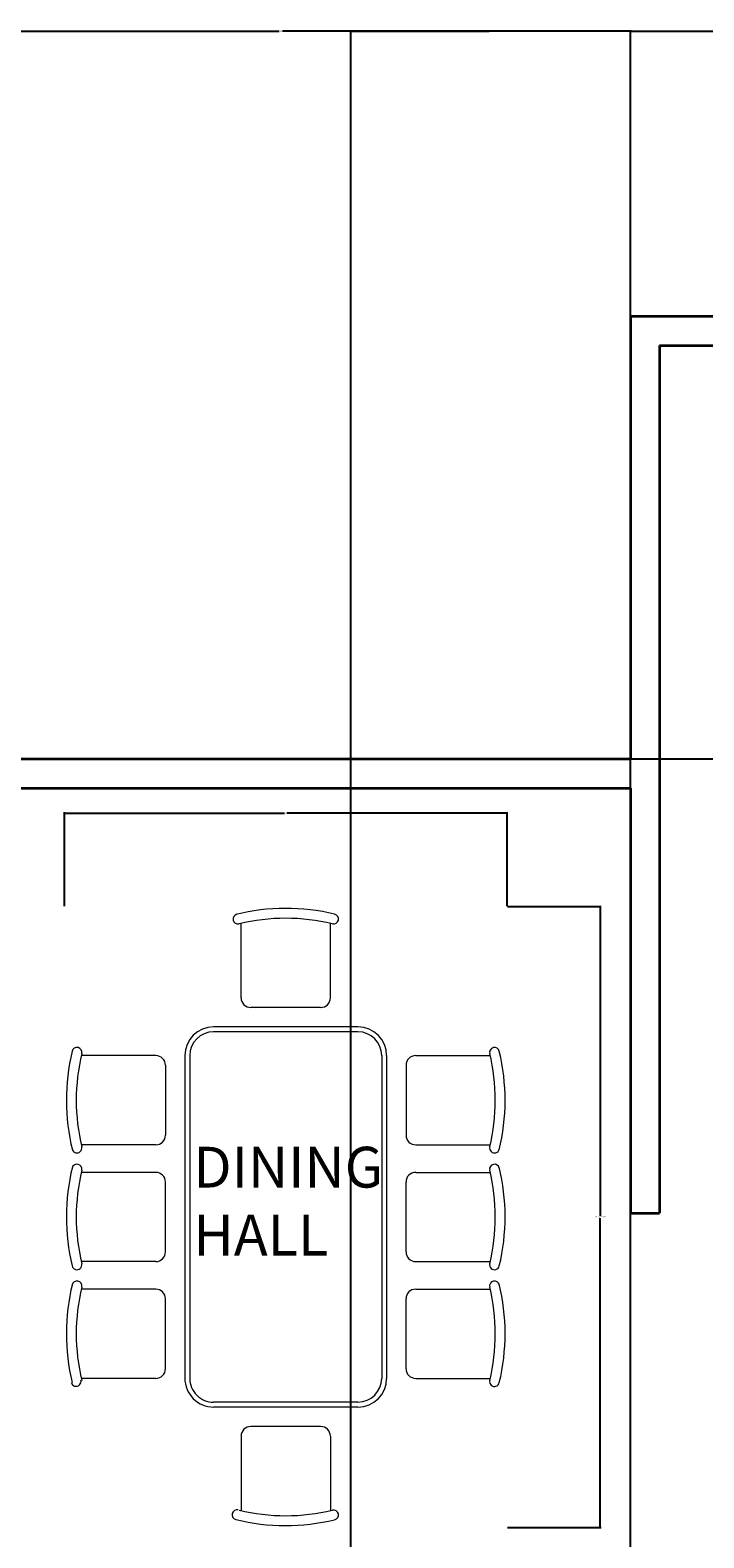
# Model space of a CAD drawing. Units: inches. Extents: x 3731 to 4318, y 1310 to 2388.
# Tile 49 of 57: x 4000 to 4116, y 2129 to 2388. Entities that reach past the tile are written whole.
import ezdxf

# ---------------------------------------------------------------- set-up
doc = ezdxf.new("R2010")
doc.units = ezdxf.units.IN
for name, color, linetype, lineweight in [('A-ANNO-DIMS', 2, 'Continuous', 18), ('A-AREA-IDEN', 7, 'Continuous', 18), ('A-FURN', 8, 'Continuous', 13), ('A-WALL', 7, 'Continuous', 35)]:
    doc.layers.add(name, color=color, linetype=linetype, lineweight=lineweight)
doc.styles.get("Standard").update_dxf_attribs({"font": 'arial.ttf'})
doc.dimstyles.get("Standard").update_dxf_attribs({"dimtxt": 0.18, "dimasz": 0.18, "dimexe": 0.18, "dimexo": 0.0625, "dimgap": 0.09, "dimtad": 0, "dimtih": 1, "dimtoh": 1, "dimdec": 4, "dimzin": 0, "dimdsep": 46, "dimtxsty": 'Standard', "dimcen": 0.09, "dimadec": 0, "dimazin": 0, "dimtfac": 1, "dimtdec": 4, "dimtofl": 0, "dimtmove": 0, "dimatfit": 3, "dimfxl": 1, "dimtolj": 1, "dimtzin": 0, "dimarcsym": 0})

# ---------------------------------------------------------------- blocks, each defined once
blk = doc.blocks.new('A$C593F2FDE')
for p, q in [((0.8501, 2.0223), (0.8501, 2.4542)), ((1.3676, 2.0223), (1.3676, 2.4542)), ((1.5273, 2.0223), (1.5273, 2.4542)), ((2.0448, 2.0223), (2.0448, 2.4542)), ((2.2045, 2.0223), (2.2045, 2.4542)), ((2.722, 2.0223), (2.722, 2.4542)), ((0.9063, 1.966), (1.3113, 1.966)), ((1.9885, 1.966), (1.5835, 1.966)), ((2.6658, 1.966), (2.2608, 1.966)), ((0.85, 1.8535), (2.722, 1.8535)), ((0.85, 1.825), (2.722, 1.825)), ((0.6835, 1.687), (0.6835, 0.85)), ((0.7121, 1.687), (0.7121, 0.85)), ((2.86, 1.687), (2.86, 0.85)), ((2.8885, 1.687), (2.8885, 0.85)), ((0.5148, 1.5273), (0.0828, 1.5273)), ((3.0573, 1.5273), (3.4892, 1.5273)), ((0.571, 1.471), (0.571, 1.066)), ((3.001, 1.471), (3.001, 1.066)), ((0.5148, 1.0098), (0.0828, 1.0098)), ((3.0573, 1.0098), (3.4892, 1.0098)), ((0.85, 0.7121), (2.722, 0.7121)), ((0.85, 0.6835), (2.722, 0.6835)), ((0.9063, 0.571), (1.3113, 0.571)), ((1.9885, 0.571), (1.5835, 0.571)), ((2.6658, 0.571), (2.2608, 0.571)), ((0.8501, 0.5148), (0.8501, 0.0828)), ((1.3676, 0.5148), (1.3676, 0.0828)), ((1.5273, 0.5148), (1.5273, 0.0828)), ((2.0448, 0.5148), (2.0448, 0.0828)), ((2.2045, 0.5148), (2.2045, 0.0828)), ((2.722, 0.5148), (2.722, 0.0828))]:
    blk.add_line(p, q)
for centre, radius, start, end in [((1.1088, 1.3263), 1.2144, 76.2483, 103.50545), ((1.786, 1.3263), 1.2144, 76.49455, 103.7517), ((2.4633, 1.3263), 1.2144, 76.49455, 103.7517), ((0.8316, 2.4793), 0.0286, 102.88207, 282.88207), ((1.1088, 1.3263), 1.1572, 76.46376, 103.53624), ((1.386, 2.4793), 0.0286, 257.11793, 77.11793), ((1.5088, 2.4793), 0.0286, 102.88207, 282.88207), ((1.786, 1.3263), 1.1572, 76.46376, 103.53624), ((2.0633, 2.4793), 0.0286, 257.11793, 77.11793), ((2.186, 2.4793), 0.0286, 102.88207, 282.88207), ((2.4633, 1.3263), 1.1572, 76.46376, 103.53624), ((2.7405, 2.4793), 0.0286, 257.11793, 77.11793), ((0.9063, 2.0223), 0.0563, 180, 270), ((1.3113, 2.0223), 0.0563, 270, 0), ((1.5835, 2.0223), 0.0563, 180, 270), ((1.9885, 2.0223), 0.0563, 270, 0), ((2.2608, 2.0223), 0.0563, 180, 270), ((2.6658, 2.0223), 0.0563, 270, 0), ((0.85, 1.687), 0.1665, 90, 180), ((2.722, 1.687), 0.1665, 0, 90), ((0.85, 1.687), 0.1379, 90, 180), ((2.722, 1.687), 0.1379, 0, 90), ((0.0578, 1.5458), 0.0286, 347.11793, 167.11793), ((3.5143, 1.5458), 0.0286, 12.88207, 192.88207), ((1.2108, 1.2685), 1.2144, 166.49455, 193.7517), ((1.2108, 1.2685), 1.1572, 166.46376, 193.53624), ((0.5148, 1.471), 0.0563, 0, 90), ((3.0573, 1.471), 0.0563, 90, 180), ((2.3613, 1.2685), 1.1572, 346.46376, 13.53624), ((2.3613, 1.2685), 1.2144, 346.2483, 13.50545), ((0.5148, 1.066), 0.0563, 270, 0), ((3.0573, 1.066), 0.0563, 180, 270), ((0.0578, 0.9913), 0.0286, 192.88207, 12.88207), ((3.513, 0.9862), 0.0286, 167.11793, 347.11793), ((0.85, 0.85), 0.1665, 180, 270), ((0.85, 0.85), 0.1379, 180, 270), ((2.722, 0.85), 0.1665, 270, 0), ((2.722, 0.85), 0.1379, 270, 0), ((0.9063, 0.5148), 0.0563, 90, 180), ((1.3113, 0.5148), 0.0563, 0, 90), ((1.5835, 0.5148), 0.0563, 90, 180), ((1.9885, 0.5148), 0.0563, 0, 90), ((2.2608, 0.5148), 0.0563, 90, 180), ((2.6658, 0.5148), 0.0563, 0, 90), ((0.8316, 0.0578), 0.0286, 77.11793, 257.11793), ((1.1088, 1.2108), 1.2144, 256.49455, 283.7517), ((1.1088, 1.2108), 1.1572, 256.46376, 283.53624), ((1.386, 0.0578), 0.0286, 282.88207, 102.88207), ((1.5088, 0.0578), 0.0286, 77.11793, 257.11793), ((1.786, 1.2108), 1.2144, 256.2483, 283.50545), ((1.786, 1.2108), 1.1572, 256.46376, 283.53624), ((2.0633, 0.0578), 0.0286, 282.88207, 102.88207), ((2.186, 0.0578), 0.0286, 77.11793, 257.11793), ((2.4633, 1.2108), 1.2144, 256.2483, 283.50545), ((2.4633, 1.2108), 1.1572, 256.46376, 283.53624), ((2.7393, 0.0528), 0.0286, 282.88207, 102.88207)]:
    blk.add_arc(centre, radius, start, end)
blk = doc.blocks.new('*D30')
at = {"layer": 'A-ANNO-DIMS', "color": 0, "lineweight": -2, "transparency": 16777216}
for p, q in [((4082.11, 2237.06), (4098.22, 2237.06)), ((4098.04, 2236.88), (4098.04, 2183.92)), ((4098.04, 2130.59), (4098.04, 2183.55)), ((4082.11, 2130.41), (4098.22, 2130.41))]:
    blk.add_line(p, q, dxfattribs=at)
at = {"layer": 'A-ANNO-DIMS', "color": 0, "transparency": 16777216}
for points in [[(4098.01, 2236.88), (4098.07, 2236.88), (4098.04, 2237.06)], [(4098.01, 2130.59), (4098.07, 2130.59), (4098.04, 2130.41)]]:
    blk.add_solid(points, dxfattribs=at)
at = {"layer": 'Defpoints', "color": 0, "transparency": 16777216}
for p in [(4082.05, 2237.06), (4082.05, 2130.41), (4098.04, 2130.41)]:
    blk.add_point(p, dxfattribs=at)
at = {"layer": 'A-ANNO-DIMS', "color": 0, "transparency": 16777216, "insert": (4098.04, 2183.74), "char_height": 0.18, "attachment_point": 5}
blk.add_mtext('\\A1;DINING SET 107', dxfattribs=at)
blk = doc.blocks.new('*D31')
at = {"layer": 'A-ANNO-DIMS', "color": 0, "lineweight": -2, "transparency": 16777216}
for p, q in [((4006.04, 2237.12), (4006.04, 2253.24)), ((4006.22, 2253.06), (4043.82, 2253.06)), ((4081.87, 2253.06), (4044.26, 2253.06)), ((4082.05, 2237.12), (4082.05, 2253.24))]:
    blk.add_line(p, q, dxfattribs=at)
at = {"layer": 'A-ANNO-DIMS', "color": 0, "transparency": 16777216}
for points in [[(4006.22, 2253.09), (4006.22, 2253.03), (4006.04, 2253.06)], [(4081.87, 2253.09), (4081.87, 2253.03), (4082.05, 2253.06)]]:
    blk.add_solid(points, dxfattribs=at)
at = {"layer": 'Defpoints', "color": 0, "transparency": 16777216}
for p in [(4082.05, 2253.06), (4006.04, 2237.06), (4082.05, 2237.06)]:
    blk.add_point(p, dxfattribs=at)
at = {"layer": 'A-ANNO-DIMS', "color": 0, "transparency": 16777216, "insert": (4044.04, 2253.06), "char_height": 0.18, "attachment_point": 5}
blk.add_mtext('\\A1;76', dxfattribs=at)
blk = doc.blocks.new('*D35')
at = {"layer": 'A-ANNO-DIMS', "color": 0, "lineweight": -2, "transparency": 16777216}
for p, q in [((3983.21, 2338.44), (3983.21, 2387.51)), ((3983.39, 2387.33), (4042.93, 2387.33)), ((4103.03, 2387.33), (4043.49, 2387.33)), ((4103.21, 2338.44), (4103.21, 2387.51))]:
    blk.add_line(p, q, dxfattribs=at)
at = {"layer": 'A-ANNO-DIMS', "color": 0, "transparency": 16777216}
for points in [[(3983.39, 2387.36), (3983.39, 2387.3), (3983.21, 2387.33)], [(4103.03, 2387.36), (4103.03, 2387.3), (4103.21, 2387.33)]]:
    blk.add_solid(points, dxfattribs=at)
at = {"layer": 'Defpoints', "color": 0, "transparency": 16777216}
for p in [(4103.21, 2387.33), (3983.21, 2338.38), (4103.21, 2338.38)]:
    blk.add_point(p, dxfattribs=at)
at = {"layer": 'A-ANNO-DIMS', "color": 0, "transparency": 16777216, "insert": (4043.21, 2387.33), "char_height": 0.18, "attachment_point": 5}
blk.add_mtext('\\A1;120', dxfattribs=at)
blk = doc.blocks.new('*D36')
at = {"layer": 'A-ANNO-DIMS', "color": 0, "lineweight": -2, "transparency": 16777216}
for p, q in [((4103.21, 2338.44), (4103.21, 2387.51)), ((4103.39, 2387.33), (4170.93, 2387.33)), ((4239.03, 2387.33), (4171.49, 2387.33)), ((4239.21, 2338.44), (4239.21, 2387.51))]:
    blk.add_line(p, q, dxfattribs=at)
at = {"layer": 'A-ANNO-DIMS', "color": 0, "transparency": 16777216}
for points in [[(4103.39, 2387.36), (4103.39, 2387.3), (4103.21, 2387.33)], [(4239.03, 2387.36), (4239.03, 2387.3), (4239.21, 2387.33)]]:
    blk.add_solid(points, dxfattribs=at)
at = {"layer": 'Defpoints', "color": 0, "transparency": 16777216}
for p in [(4239.21, 2387.33), (4103.21, 2338.38), (4239.21, 2338.38)]:
    blk.add_point(p, dxfattribs=at)
at = {"layer": 'A-ANNO-DIMS', "color": 0, "transparency": 16777216, "insert": (4171.21, 2387.33), "char_height": 0.18, "attachment_point": 5}
blk.add_mtext('\\A1;136', dxfattribs=at)
blk = doc.blocks.new('*D37')
at = {"layer": 'A-ANNO-DIMS', "color": 0, "lineweight": -2, "transparency": 16777216}
for p, q in [((4239.27, 2338.38), (4318.34, 2338.38)), ((4318.16, 2338.2), (4318.16, 2300.56)), ((4318.16, 2262.56), (4318.16, 2300.2)), ((4103.27, 2262.38), (4318.34, 2262.38))]:
    blk.add_line(p, q, dxfattribs=at)
at = {"layer": 'A-ANNO-DIMS', "color": 0, "transparency": 16777216}
for points in [[(4318.13, 2338.2), (4318.19, 2338.2), (4318.16, 2338.38)], [(4318.13, 2262.56), (4318.19, 2262.56), (4318.16, 2262.38)]]:
    blk.add_solid(points, dxfattribs=at)
at = {"layer": 'Defpoints', "color": 0, "transparency": 16777216}
for p in [(4239.21, 2338.38), (4318.16, 2338.38), (4103.21, 2262.38)]:
    blk.add_point(p, dxfattribs=at)
at = {"layer": 'A-ANNO-DIMS', "color": 0, "transparency": 16777216, "insert": (4318.16, 2300.38), "char_height": 0.18, "attachment_point": 5}
blk.add_mtext('\\A1;76', dxfattribs=at)
blk = doc.blocks.new('*D38')
at = {"layer": 'A-ANNO-DIMS', "color": 0, "lineweight": -2, "transparency": 16777216}
for p, q in [((4103.27, 2262.38), (4318.34, 2262.38)), ((4318.16, 2262.2), (4318.16, 2103.06)), ((4318.16, 1943.56), (4318.16, 2102.7)), ((4234.27, 1943.38), (4318.34, 1943.38))]:
    blk.add_line(p, q, dxfattribs=at)
at = {"layer": 'A-ANNO-DIMS', "color": 0, "transparency": 16777216}
for points in [[(4318.13, 2262.2), (4318.19, 2262.2), (4318.16, 2262.38)], [(4318.13, 1943.56), (4318.19, 1943.56), (4318.16, 1943.38)]]:
    blk.add_solid(points, dxfattribs=at)
at = {"layer": 'Defpoints', "color": 0, "transparency": 16777216}
for p in [(4103.21, 2262.38), (4318.16, 2262.38), (4234.21, 1943.38)]:
    blk.add_point(p, dxfattribs=at)
at = {"layer": 'A-ANNO-DIMS', "color": 0, "transparency": 16777216, "insert": (4318.16, 2102.88), "char_height": 0.18, "attachment_point": 5}
blk.add_mtext('\\A1;319', dxfattribs=at)
blk = doc.blocks.new('*D49')
at = {"layer": 'A-ANNO-DIMS', "color": 0, "lineweight": -2, "transparency": 16777216}
for p, q in [((4055.21, 1943.44), (4055.21, 2387.51)), ((4055.39, 2387.33), (4078.99, 2387.33)), ((4103.03, 2387.33), (4079.43, 2387.33)), ((4103.21, 1938.44), (4103.21, 2387.51))]:
    blk.add_line(p, q, dxfattribs=at)
at = {"layer": 'A-ANNO-DIMS', "color": 0, "transparency": 16777216}
for points in [[(4055.39, 2387.36), (4055.39, 2387.3), (4055.21, 2387.33)], [(4103.03, 2387.36), (4103.03, 2387.3), (4103.21, 2387.33)]]:
    blk.add_solid(points, dxfattribs=at)
at = {"layer": 'Defpoints', "color": 0, "transparency": 16777216}
for p in [(4103.21, 2387.33), (4055.21, 1943.38), (4103.21, 1938.38)]:
    blk.add_point(p, dxfattribs=at)
at = {"layer": 'A-ANNO-DIMS', "color": 0, "transparency": 16777216, "insert": (4079.21, 2387.33), "char_height": 0.18, "attachment_point": 5}
blk.add_mtext('\\A1;48', dxfattribs=at)

msp = doc.modelspace()

# ---------------------------------------------------------------- linework, layer by layer
at = {"layer": 'A-WALL'}
for p, q in [((4103.21, 2338.38), (4103.21, 2262.38)), ((4103.21, 2338.38), (4239.21, 2338.38)), ((4108.21, 2333.38), (4108.21, 2184.38)), ((4108.21, 2333.38), (4234.21, 2333.38)), ((3983.21, 2262.38), (4103.21, 2262.38)), ((3983.21, 2257.38), (4103.21, 2257.38)), ((4103.21, 2257.38), (4103.21, 2184.38)), ((4103.21, 2184.38), (4108.21, 2184.38))]:
    msp.add_line(p, q, dxfattribs=at)

# ---------------------------------------------------------------- block references
at = {"layer": 'A-FURN', "xscale": 29.60417329027022, "yscale": 29.60417329027022, "zscale": 29.60417329027022, "rotation": 270}
msp.add_blockref('A$C593F2FDE', (4006.49, 2236.61), dxfattribs=at)

# ---------------------------------------------------------------- texts
at = {"layer": 'A-AREA-IDEN', "insert": (4028.19, 2195.79), "char_height": 7, "attachment_point": 1}
msp.add_mtext_dynamic_manual_height_columns('DINING\\PHALL', width=24.0878, gutter_width=12.5, heights=[0], dxfattribs=at)

# ---------------------------------------------------------------- dimensions: what is measured, and where the dimension line sits
at = {"layer": 'A-ANNO-DIMS'}
for base, p1, p2, picture, middle in [((4103.21, 2387.33), (3983.21, 2338.38), (4103.21, 2338.38), '*D35', (4043.21, 2387.33)), ((4103.21, 2387.33), (4055.21, 1943.38), (4103.21, 1938.38), '*D49', (4079.21, 2387.33)), ((4239.21, 2387.33), (4103.21, 2338.38), (4239.21, 2338.38), '*D36', (4171.21, 2387.33)), ((4082.05, 2253.06), (4006.04, 2237.06), (4082.05, 2237.06), '*D31', (4044.04, 2253.06))]:
    dim = msp.add_linear_dim(base=base, p1=p1, p2=p2, dimstyle='Standard', override={"dimdec": 0, "dimlfac": 1, "dimrnd": 0, "dimzin": 0, "dimdsep": 46, "dimlunit": 2}, dxfattribs=at)
    dim.commit()
    dim.dimension.update_dxf_attribs({"geometry": picture, "text_midpoint": middle})
for base, p1, p2, picture, middle in [((4318.16, 2338.38), (4103.21, 2262.38), (4239.21, 2338.38), '*D37', (4318.16, 2300.38)), ((4318.16, 2262.38), (4234.21, 1943.38), (4103.21, 2262.38), '*D38', (4318.16, 2102.88))]:
    dim = msp.add_linear_dim(base=base, p1=p1, p2=p2, angle=90, dimstyle='Standard', override={"dimdec": 0, "dimlfac": 1, "dimrnd": 0, "dimzin": 0, "dimdsep": 46, "dimlunit": 2}, dxfattribs=at)
    dim.commit()
    dim.dimension.update_dxf_attribs({"geometry": picture, "text_midpoint": middle})
dim = msp.add_linear_dim(base=(4098.04, 2130.41), p1=(4082.05, 2237.06), p2=(4082.05, 2130.41), angle=270, text='DINING SET <>', dimstyle='Standard', override={"dimdec": 0, "dimlfac": 1, "dimrnd": 0, "dimzin": 0, "dimdsep": 46, "dimlunit": 2}, dxfattribs=at)
dim.commit()
dim.dimension.update_dxf_attribs({"geometry": '*D30', "text_midpoint": (4098.04, 2183.74)})

doc.saveas('drawing.dxf')
